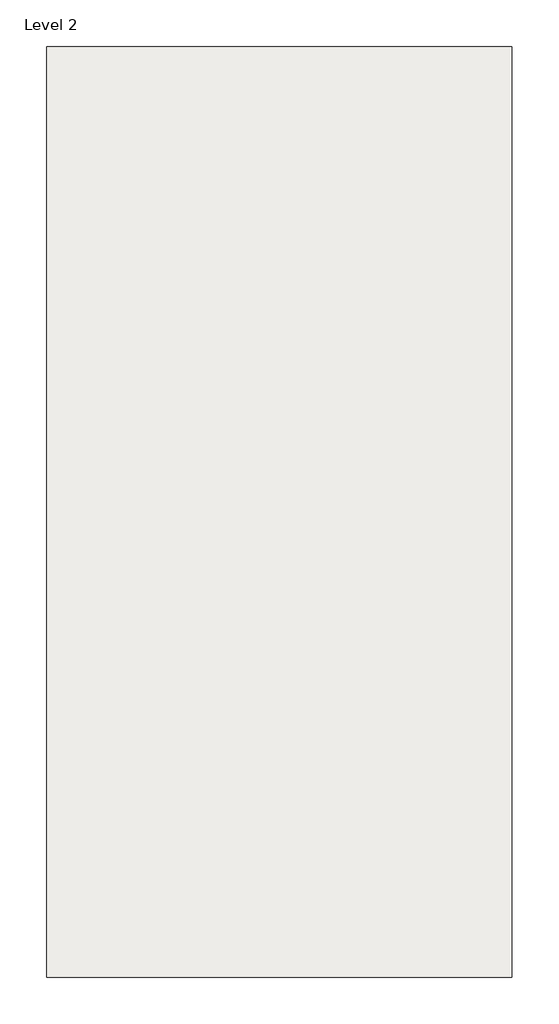
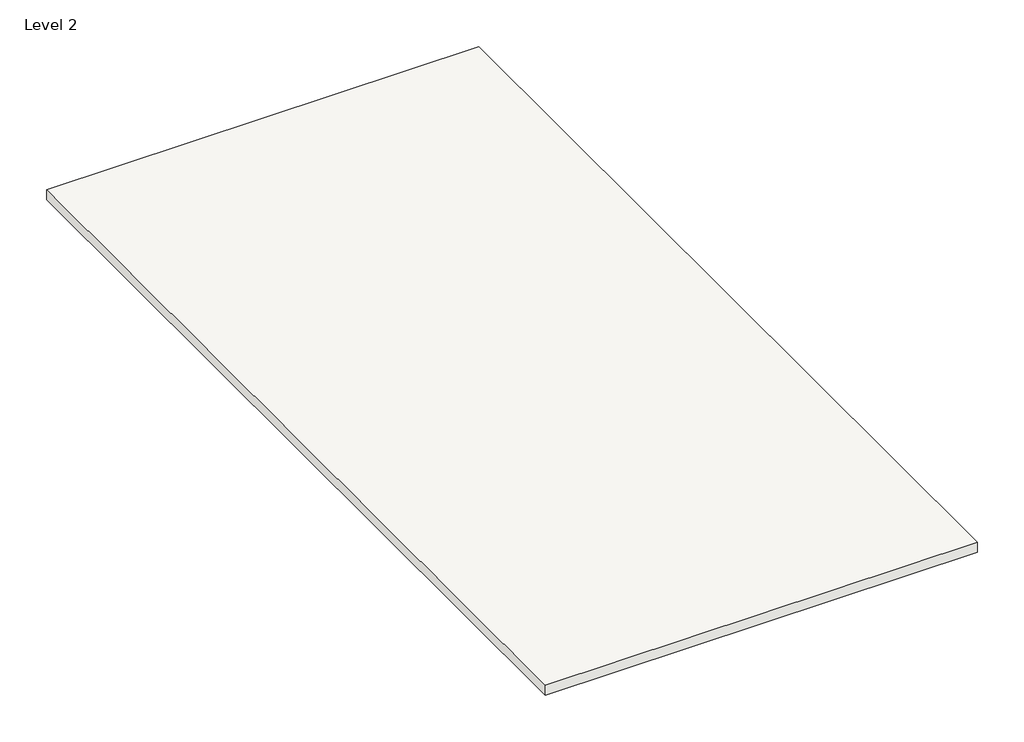
# One storey: 1 roof.
"""IFC4 building model written with IfcOpenShell, lengths in millimetres."""

from ifc_helpers import new_model, si_unit, frame, origin, place, context, project, spatial, polyline, outline, extrude, element, save

model = new_model("IFC4")

# Units and contexts
model_context = context("Model", 3, world=origin())
ifc_project = project(units=[si_unit("LENGTHUNIT", "METRE", prefix="MILLI")], contexts=[model_context])

# Site, building, storey
site = spatial("IfcSite", under=ifc_project)
building = spatial("IfcBuilding", under=site)
storey = spatial("IfcBuildingStorey", under=building, Name="Level 2", Elevation=3048.0)

# Roof
placement = place(None, origin())
element("IfcRoof", 1, ObjectType="Generic - 12\"", at=placement, inside=storey, context=model_context, shape_type="SweptSolid", body=[
    extrude(outline(polyline([(1524.0, 14224.0), (7620.0, 14224.0), (7620.0, 2032.0), (1524.0, 2032.0), (1524.0, 14224.0)])), frame((0.0, 0.0, 3048.0), z_axis=(0.0, 0.0, 1.0), x_axis=(1.0, 0.0, 0.0)), (0.0, 0.0, 1.0), 152.4),
])

save(model, "model.ifc")

# Revit data of these elements
# Type "Generic - 12\""
#   Assembly Code = "B1020"
#   Layers, outside or top first: 0' - 6" "Plywood, Sheathing" (function 1)
# Element 1 (IfcRoof, "Generic - 12\"")
#   built-in parameter 1001705 = 10.5 (stored number, unit not read)
#   built-in parameter 1001710 = 33615
#   Phase Created = New Construction
#   Materials on its faces: "Plywood, Sheathing"
# Materials
#   "Plywood, Sheathing": class "Wood", colour RGB 212 179 113, transparency 0, Description = "Plywood, sheathing grade", Cost = 0
